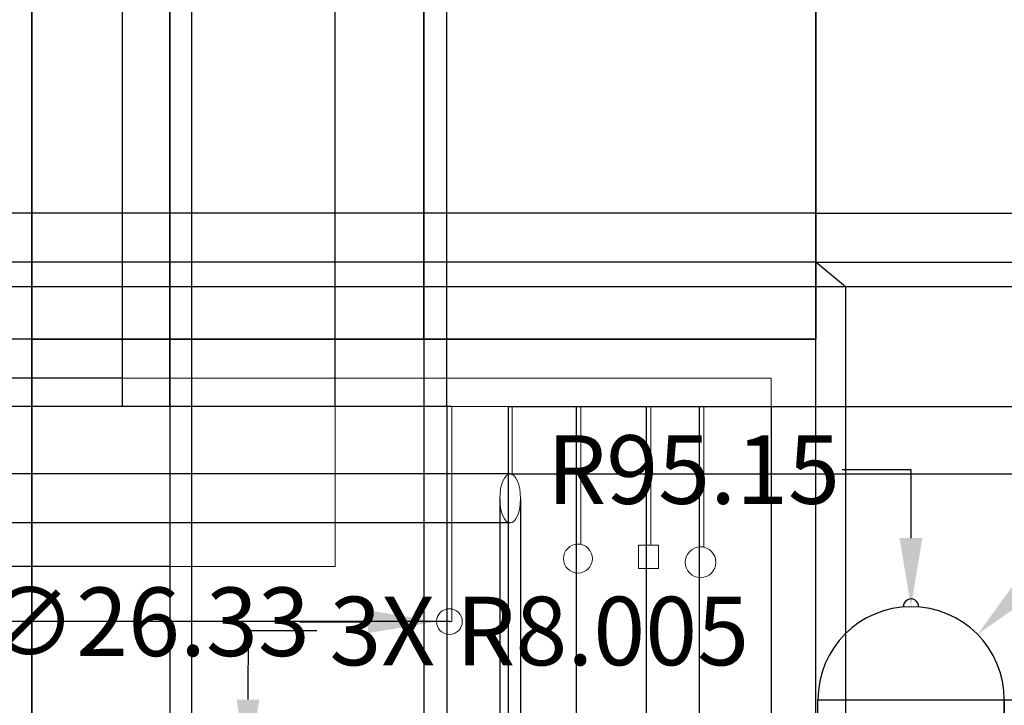
# Model space of a CAD drawing. Units: inches. Extents: x 600 to 5582, y -464 to 3142.
# Tile 4 of 9: x 1772 to 2777, y 1229 to 1928. Entities that reach past the tile are written whole.
import ezdxf

# ---------------------------------------------------------------- set-up
doc = ezdxf.new("R2010")
doc.units = ezdxf.units.IN
doc.header["$MEASUREMENT"] = 0
for name, color, linetype, lineweight in [('A-ANNO-DIMS', 2, 'Continuous', 18), ('A-ELEV', 7, 'Continuous', 35), ('A-ELEV-PATT', 252, 'Continuous', 13), ('A-EQPM', 4, 'Continuous', 25), ('A-FURN', 8, 'Continuous', 18)]:
    doc.layers.add(name, color=color, linetype=linetype, lineweight=lineweight)
doc.styles.get("Standard").update_dxf_attribs({"font": 'arial.ttf'})
doc.dimstyles.get("Standard").update_dxf_attribs({"dimtxt": 70, "dimasz": 70, "dimexe": 0.18, "dimexo": 0.0625, "dimgap": 0.09, "dimtad": 0, "dimtih": 1, "dimtoh": 1, "dimdec": 0, "dimzin": 0, "dimdsep": 46, "dimtxsty": 'Standard', "dimcen": 0.09, "dimadec": 0, "dimazin": 0, "dimtfac": 1, "dimtdec": 0, "dimtofl": 0, "dimtmove": 0, "dimatfit": 3, "dimfxl": 1, "dimtolj": 1, "dimtzin": 0, "dimarcsym": 0})

# ---------------------------------------------------------------- blocks, each defined once
blk = doc.blocks.new('*D22')
at = {"layer": 'A-ANNO-DIMS', "color": 0, "lineweight": -2, "transparency": 16777216}
for p, q in [((1149.2, 1725.8), (1149.2, 1795.8)), ((2615, 1655.8), (1149.1, 1655.8)), ((2584.7, 1602.4), (1149.1, 1602.4)), ((1149.2, 1532.4), (1149.2, 1462.4)), ((1149.2, 1462.4), (1079.2, 1462.4))]:
    blk.add_line(p, q, dxfattribs=at)
at = {"layer": 'A-ANNO-DIMS', "color": 0, "transparency": 16777216}
for points in [[(1137.6, 1725.8), (1160.9, 1725.8), (1149.2, 1655.8)], [(1137.6, 1532.4), (1160.9, 1532.4), (1149.2, 1602.4)]]:
    blk.add_solid(points, dxfattribs=at)
at = {"layer": 'Defpoints', "color": 0, "transparency": 16777216}
for p in [(2615, 1655.8), (1149.2, 1602.4), (2584.7, 1602.4)]:
    blk.add_point(p, dxfattribs=at)
at = {"layer": 'A-ANNO-DIMS', "color": 0, "transparency": 16777216, "insert": (967.8, 1462.4), "char_height": 70, "attachment_point": 5}
blk.add_mtext('\\A1;53.41', dxfattribs=at)
blk = doc.blocks.new('*D23')
at = {"layer": 'A-ANNO-DIMS', "color": 0, "lineweight": -2, "transparency": 16777216}
for p, q in [((1149.2, 1750.8), (1149.2, 1820.8)), ((1149.2, 1820.8), (1219.2, 1820.8)), ((2584.7, 1680.8), (1149.1, 1680.8)), ((2615, 1655.8), (1149.1, 1655.8)), ((1149.2, 1585.8), (1149.2, 1515.8))]:
    blk.add_line(p, q, dxfattribs=at)
at = {"layer": 'A-ANNO-DIMS', "color": 0, "transparency": 16777216}
for points in [[(1137.6, 1750.8), (1160.9, 1750.8), (1149.2, 1680.8)], [(1137.6, 1585.8), (1160.9, 1585.8), (1149.2, 1655.8)]]:
    blk.add_solid(points, dxfattribs=at)
at = {"layer": 'Defpoints', "color": 0, "transparency": 16777216}
for p in [(1149.2, 1680.8), (2584.7, 1680.8), (2615, 1655.8)]:
    blk.add_point(p, dxfattribs=at)
at = {"layer": 'A-ANNO-DIMS', "color": 0, "transparency": 16777216, "insert": (1270.3, 1820.8), "char_height": 70, "attachment_point": 5}
blk.add_mtext('\\A1;25', dxfattribs=at)
blk = doc.blocks.new('*D24')
at = {"layer": 'A-ANNO-DIMS', "color": 0, "lineweight": -2, "transparency": 16777216}
for p, q in [((1149.2, 1800.8), (1149.2, 1870.8)), ((1149.2, 1870.8), (1219.2, 1870.8)), ((2584.7, 1730.8), (1149.1, 1730.8)), ((2584.7, 1680.8), (1149.1, 1680.8)), ((1149.2, 1610.8), (1149.2, 1540.8))]:
    blk.add_line(p, q, dxfattribs=at)
at = {"layer": 'A-ANNO-DIMS', "color": 0, "transparency": 16777216}
for points in [[(1137.6, 1800.8), (1160.9, 1800.8), (1149.2, 1730.8)], [(1137.6, 1610.8), (1160.9, 1610.8), (1149.2, 1680.8)]]:
    blk.add_solid(points, dxfattribs=at)
at = {"layer": 'Defpoints', "color": 0, "transparency": 16777216}
for p in [(1149.2, 1730.8), (2584.7, 1730.8), (2584.7, 1680.8)]:
    blk.add_point(p, dxfattribs=at)
at = {"layer": 'A-ANNO-DIMS', "color": 0, "transparency": 16777216, "insert": (1269.4, 1870.8), "char_height": 70, "attachment_point": 5}
blk.add_mtext('\\A1;50', dxfattribs=at)
blk = doc.blocks.new('*D25')
at = {"layer": 'A-ANNO-DIMS', "color": 0, "lineweight": -2, "transparency": 16777216}
for p, q in [((2584.7, 1680.8), (2584.7, -233.3)), ((2615, 1655.8), (2615, -233.3)), ((2514.7, -233.1), (2444.7, -233.1)), ((2685, -233.1), (2755, -233.1))]:
    blk.add_line(p, q, dxfattribs=at)
at = {"layer": 'A-ANNO-DIMS', "color": 0, "transparency": 16777216}
for points in [[(2514.7, -221.4), (2514.7, -244.7), (2584.7, -233.1)], [(2685, -221.4), (2685, -244.7), (2615, -233.1)]]:
    blk.add_solid(points, dxfattribs=at)
at = {"layer": 'Defpoints', "color": 0, "transparency": 16777216}
for p in [(2584.7, 1680.8), (2615, 1655.8), (2615, -233.1)]:
    blk.add_point(p, dxfattribs=at)
at = {"layer": 'A-ANNO-DIMS', "color": 0, "transparency": 16777216, "insert": (2873.3, -233.1), "char_height": 70, "attachment_point": 5}
blk.add_mtext('\\A1;30.28', dxfattribs=at)
blk = doc.blocks.new('*D59')
at = {"layer": 'A-ANNO-DIMS', "color": 0, "lineweight": -2, "transparency": 16777216}
for p, q in [((2611.9, 1469.2), (2681.9, 1469.2)), ((2681.9, 1469.2), (2681.9, 1399.2)), ((2682, 1234), (2682.2, 1234)), ((2682.1, 1234), (2682.1, 1234.1))]:
    blk.add_line(p, q, dxfattribs=at)
at = {"layer": 'A-ANNO-DIMS', "color": 0, "transparency": 16777216}
blk.add_solid([(2693.6, 1399.2), (2670.3, 1399.2), (2682, 1329.2)], dxfattribs=at)
at = {"layer": 'Defpoints', "color": 0, "transparency": 16777216}
for p in [(2682, 1329.2), (2682.1, 1234)]:
    blk.add_point(p, dxfattribs=at)
at = {"layer": 'A-ANNO-DIMS', "color": 0, "transparency": 16777216, "insert": (2459.9, 1469.2), "char_height": 70, "attachment_point": 5}
blk.add_mtext('\\A1;R95.15', dxfattribs=at)
blk = doc.blocks.new('*D63')
at = {"layer": 'A-ANNO-DIMS', "color": 0, "lineweight": -2, "transparency": 16777216}
for p, q in [((2584.7, 2352.4), (1149.1, 2352.4)), ((1149.2, 2282.4), (1149.2, 2077.5)), ((1149.2, 1800.8), (1149.2, 2005.8)), ((2584.7, 1730.8), (1149.1, 1730.8))]:
    blk.add_line(p, q, dxfattribs=at)
at = {"layer": 'A-ANNO-DIMS', "color": 0, "transparency": 16777216}
for points in [[(1137.6, 2282.4), (1160.9, 2282.4), (1149.2, 2352.4)], [(1137.6, 1800.8), (1160.9, 1800.8), (1149.2, 1730.8)]]:
    blk.add_solid(points, dxfattribs=at)
at = {"layer": 'Defpoints', "color": 0, "transparency": 16777216}
for p in [(1149.2, 2352.4), (2584.7, 2352.4), (2584.7, 1730.8)]:
    blk.add_point(p, dxfattribs=at)
at = {"layer": 'A-ANNO-DIMS', "color": 0, "transparency": 16777216, "insert": (1149.2, 2041.6), "char_height": 70, "attachment_point": 5}
blk.add_mtext('\\A1;621.59', dxfattribs=at)
blk = doc.blocks.new('*D65')
at = {"layer": 'A-ANNO-DIMS', "color": 0, "lineweight": -2, "transparency": 16777216}
for p, q in [((1784.7, 2352.4), (1784.7, -233.3)), ((2184.7, 2352.4), (2184.7, -233.3)), ((1714.7, -233.1), (1644.7, -233.1)), ((2254.7, -233.1), (2324.7, -233.1))]:
    blk.add_line(p, q, dxfattribs=at)
at = {"layer": 'A-ANNO-DIMS', "color": 0, "transparency": 16777216}
for points in [[(1714.7, -221.4), (1714.7, -244.7), (1784.7, -233.1)], [(2254.7, -221.4), (2254.7, -244.7), (2184.7, -233.1)]]:
    blk.add_solid(points, dxfattribs=at)
at = {"layer": 'Defpoints', "color": 0, "transparency": 16777216}
for p in [(1784.7, 2352.4), (2184.7, 2352.4), (2184.7, -233.1)]:
    blk.add_point(p, dxfattribs=at)
at = {"layer": 'A-ANNO-DIMS', "color": 0, "transparency": 16777216, "insert": (1984.7, -233.1), "char_height": 70, "attachment_point": 5}
blk.add_mtext('\\A1;400.00', dxfattribs=at)
blk = doc.blocks.new('*D70')
at = {"layer": 'A-ANNO-DIMS', "color": 0, "lineweight": -2, "transparency": 16777216}
for p, q in [((1149.2, 1176.8), (1149.2, 1246.8)), ((1149.2, 1246.8), (1219.2, 1246.8)), ((2586.9, 1106.8), (1149.1, 1106.8)), ((2599.2, 1042.4), (1149.1, 1042.4)), ((1149.2, 972.4), (1149.2, 902.4))]:
    blk.add_line(p, q, dxfattribs=at)
at = {"layer": 'A-ANNO-DIMS', "color": 0, "transparency": 16777216}
for points in [[(1137.6, 1176.8), (1160.9, 1176.8), (1149.2, 1106.8)], [(1137.6, 972.4), (1160.9, 972.4), (1149.2, 1042.4)]]:
    blk.add_solid(points, dxfattribs=at)
at = {"layer": 'Defpoints', "color": 0, "transparency": 16777216}
for p in [(1149.2, 1106.8), (2586.9, 1106.8), (2599.2, 1042.4)]:
    blk.add_point(p, dxfattribs=at)
at = {"layer": 'A-ANNO-DIMS', "color": 0, "transparency": 16777216, "insert": (1337.3, 1246.8), "char_height": 70, "attachment_point": 5}
blk.add_mtext('\\A1;64.42', dxfattribs=at)
blk = doc.blocks.new('*D79')
at = {"layer": 'A-ANNO-DIMS', "color": 0, "lineweight": -2, "transparency": 16777216}
for p, q in [((1855.7, 2987.9), (1785.7, 2987.9)), ((1925.7, 1126.2), (1925.7, 2988.1)), ((1947.9, 1126.2), (1947.9, 2988.1)), ((2017.9, 2987.9), (2087.9, 2987.9))]:
    blk.add_line(p, q, dxfattribs=at)
at = {"layer": 'A-ANNO-DIMS', "color": 0, "transparency": 16777216}
for points in [[(1855.7, 2999.6), (1855.7, 2976.3), (1925.7, 2987.9)], [(2017.9, 2999.6), (2017.9, 2976.3), (1947.9, 2987.9)]]:
    blk.add_solid(points, dxfattribs=at)
at = {"layer": 'Defpoints', "color": 0, "transparency": 16777216}
for p in [(1947.9, 2987.9), (1925.7, 1126.1), (1947.9, 1126.1)]:
    blk.add_point(p, dxfattribs=at)
at = {"layer": 'A-ANNO-DIMS', "color": 0, "transparency": 16777216, "insert": (2234.2, 2987.9), "char_height": 70, "attachment_point": 5}
blk.add_mtext('\\A1;22.235', dxfattribs=at)
blk = doc.blocks.new('*D80')
at = {"layer": 'A-ANNO-DIMS', "color": 0, "lineweight": -2, "transparency": 16777216}
for p, q in [((1149.2, 1196.1), (1149.2, 1266.1)), ((1925.6, 1126.1), (1149.1, 1126.1)), ((1925.6, 1042.4), (1149.1, 1042.4)), ((1149.2, 972.4), (1149.2, 902.4))]:
    blk.add_line(p, q, dxfattribs=at)
at = {"layer": 'A-ANNO-DIMS', "color": 0, "transparency": 16777216}
for points in [[(1137.6, 1196.1), (1160.9, 1196.1), (1149.2, 1126.1)], [(1137.6, 972.4), (1160.9, 972.4), (1149.2, 1042.4)]]:
    blk.add_solid(points, dxfattribs=at)
at = {"layer": 'Defpoints', "color": 0, "transparency": 16777216}
for p in [(1149.2, 1126.1), (1925.7, 1126.1), (1925.7, 1042.4)]:
    blk.add_point(p, dxfattribs=at)
at = {"layer": 'A-ANNO-DIMS', "color": 0, "transparency": 16777216, "insert": (1149.2, 1084.3), "char_height": 70, "attachment_point": 5}
blk.add_mtext('\\A1;83.69', dxfattribs=at)
blk = doc.blocks.new('*D81')
at = {"layer": 'A-ANNO-DIMS', "color": 0, "lineweight": -2, "transparency": 16777216}
for p, q in [((5220.2, 1133.7), (5220.2, 1203.7)), ((5220.2, 1203.7), (5290.2, 1203.7)), ((2292.1, 1063.7), (5220.4, 1063.7)), ((2310.1, 1042.4), (5220.4, 1042.4)), ((5220.2, 972.4), (5220.2, 902.4))]:
    blk.add_line(p, q, dxfattribs=at)
at = {"layer": 'A-ANNO-DIMS', "color": 0, "transparency": 16777216}
for points in [[(5208.6, 1133.7), (5231.9, 1133.7), (5220.2, 1063.7)], [(5208.6, 972.4), (5231.9, 972.4), (5220.2, 1042.4)]]:
    blk.add_solid(points, dxfattribs=at)
at = {"layer": 'Defpoints', "color": 0, "transparency": 16777216}
for p in [(2292, 1063.7), (5220.2, 1063.7), (2310, 1042.4)]:
    blk.add_point(p, dxfattribs=at)
at = {"layer": 'A-ANNO-DIMS', "color": 0, "transparency": 16777216, "insert": (5409, 1203.7), "char_height": 70, "attachment_point": 5}
blk.add_mtext('\\A1;21.26', dxfattribs=at)
blk = doc.blocks.new('*D85')
at = {"layer": 'A-ANNO-DIMS', "color": 0, "lineweight": -2, "transparency": 16777216}
for p, q in [((5220.2, 1193.3), (5220.2, 1263.3)), ((5220.2, 1263.3), (5290.2, 1263.3)), ((2231.9, 1123.3), (5220.4, 1123.3)), ((2232.3, 1063.4), (5220.4, 1063.4)), ((5220.2, 993.4), (5220.2, 923.4))]:
    blk.add_line(p, q, dxfattribs=at)
at = {"layer": 'A-ANNO-DIMS', "color": 0, "transparency": 16777216}
for points in [[(5208.6, 1193.3), (5231.9, 1193.3), (5220.2, 1123.3)], [(5208.6, 993.4), (5231.9, 993.4), (5220.2, 1063.4)]]:
    blk.add_solid(points, dxfattribs=at)
at = {"layer": 'Defpoints', "color": 0, "transparency": 16777216}
for p in [(2231.8, 1123.3), (5220.2, 1123.3), (2232.2, 1063.4)]:
    blk.add_point(p, dxfattribs=at)
at = {"layer": 'A-ANNO-DIMS', "color": 0, "transparency": 16777216, "insert": (5408.5, 1263.3), "char_height": 70, "attachment_point": 5}
blk.add_mtext('\\A1;59.99', dxfattribs=at)
blk = doc.blocks.new('*D86')
at = {"layer": 'A-ANNO-DIMS', "color": 0, "lineweight": -2, "transparency": 16777216}
for p, q in [((1714.7, 2987.9), (1644.7, 2987.9)), ((1784.7, 1602.5), (1784.7, 2988.1)), ((1877.2, 1562.7), (1877.2, 2988.1)), ((1947.2, 2987.9), (2017.2, 2987.9))]:
    blk.add_line(p, q, dxfattribs=at)
at = {"layer": 'A-ANNO-DIMS', "color": 0, "transparency": 16777216}
for points in [[(1714.7, 2999.6), (1714.7, 2976.3), (1784.7, 2987.9)], [(1947.2, 2999.6), (1947.2, 2976.3), (1877.2, 2987.9)]]:
    blk.add_solid(points, dxfattribs=at)
at = {"layer": 'Defpoints', "color": 0, "transparency": 16777216}
for p in [(1877.2, 2987.9), (1784.7, 1602.4), (1877.2, 1562.6)]:
    blk.add_point(p, dxfattribs=at)
at = {"layer": 'A-ANNO-DIMS', "color": 0, "transparency": 16777216, "insert": (2135.4, 2987.9), "char_height": 70, "attachment_point": 5}
blk.add_mtext('\\A1;92.46', dxfattribs=at)
blk = doc.blocks.new('*D87')
at = {"layer": 'A-ANNO-DIMS', "color": 0, "lineweight": -2, "transparency": 16777216}
for p, q in [((1149.2, 1672.4), (1149.2, 1742.4)), ((1149.2, 1742.4), (1219.2, 1742.4)), ((1784.7, 1602.4), (1149.1, 1602.4)), ((1877.1, 1562.6), (1149.1, 1562.6)), ((1149.2, 1492.6), (1149.2, 1422.6))]:
    blk.add_line(p, q, dxfattribs=at)
at = {"layer": 'A-ANNO-DIMS', "color": 0, "transparency": 16777216}
for points in [[(1137.6, 1672.4), (1160.9, 1672.4), (1149.2, 1602.4)], [(1137.6, 1492.6), (1160.9, 1492.6), (1149.2, 1562.6)]]:
    blk.add_solid(points, dxfattribs=at)
at = {"layer": 'Defpoints', "color": 0, "transparency": 16777216}
for p in [(1149.2, 1602.4), (1784.7, 1602.4), (1877.2, 1562.6)]:
    blk.add_point(p, dxfattribs=at)
at = {"layer": 'A-ANNO-DIMS', "color": 0, "transparency": 16777216, "insert": (1337.3, 1742.4), "char_height": 70, "attachment_point": 5}
blk.add_mtext('\\A1;39.80', dxfattribs=at)
blk = doc.blocks.new('*D88')
at = {"layer": 'A-ANNO-DIMS', "color": 0, "lineweight": -2, "transparency": 16777216}
for p, q in [((1149.2, 1632.6), (1149.2, 1702.6)), ((1149.2, 1702.6), (1219.2, 1702.6)), ((1877.1, 1562.6), (1149.1, 1562.6)), ((1877.1, 1533.5), (1149.1, 1533.5)), ((1149.2, 1463.5), (1149.2, 1393.5))]:
    blk.add_line(p, q, dxfattribs=at)
at = {"layer": 'A-ANNO-DIMS', "color": 0, "transparency": 16777216}
for points in [[(1137.6, 1632.6), (1160.9, 1632.6), (1149.2, 1562.6)], [(1137.6, 1463.5), (1160.9, 1463.5), (1149.2, 1533.5)]]:
    blk.add_solid(points, dxfattribs=at)
at = {"layer": 'Defpoints', "color": 0, "transparency": 16777216}
for p in [(1149.2, 1562.6), (1877.2, 1562.6), (1877.2, 1533.5)]:
    blk.add_point(p, dxfattribs=at)
at = {"layer": 'A-ANNO-DIMS', "color": 0, "transparency": 16777216, "insert": (1365.2, 1702.6), "char_height": 70, "attachment_point": 5}
blk.add_mtext('\\A1;29.136', dxfattribs=at)
blk = doc.blocks.new('*D89')
at = {"layer": 'A-ANNO-DIMS', "color": 0, "lineweight": -2, "transparency": 16777216}
for p, q in [((1807.2, 2987.9), (1737.2, 2987.9)), ((1877.2, 1533.5), (1877.2, 2988.1)), ((1925.6, 1533.5), (1925.6, 2988.1)), ((1995.6, 2987.9), (2065.6, 2987.9))]:
    blk.add_line(p, q, dxfattribs=at)
at = {"layer": 'A-ANNO-DIMS', "color": 0, "transparency": 16777216}
for points in [[(1807.2, 2999.6), (1807.2, 2976.3), (1877.2, 2987.9)], [(1995.6, 2999.6), (1995.6, 2976.3), (1925.6, 2987.9)]]:
    blk.add_solid(points, dxfattribs=at)
at = {"layer": 'Defpoints', "color": 0, "transparency": 16777216}
for p in [(1925.6, 2987.9), (1877.2, 1533.5), (1925.6, 1533.5)]:
    blk.add_point(p, dxfattribs=at)
at = {"layer": 'A-ANNO-DIMS', "color": 0, "transparency": 16777216, "insert": (2185.1, 2987.9), "char_height": 70, "attachment_point": 5}
blk.add_mtext('\\A1;48.40', dxfattribs=at)
blk = doc.blocks.new('*D90')
at = {"layer": 'A-ANNO-DIMS', "color": 0, "lineweight": -2, "transparency": 16777216}
for p, q in [((1925.6, 1533.5), (1925.6, 2988.1)), ((1995.6, 2987.9), (2024.2, 2987.9)), ((2094.2, 1533.5), (2094.2, 2988.1)), ((2094.2, 2987.9), (2164.2, 2987.9))]:
    blk.add_line(p, q, dxfattribs=at)
at = {"layer": 'A-ANNO-DIMS', "color": 0, "transparency": 16777216}
for points in [[(1995.6, 2999.6), (1995.6, 2976.3), (1925.6, 2987.9)], [(2024.2, 2999.6), (2024.2, 2976.3), (2094.2, 2987.9)]]:
    blk.add_solid(points, dxfattribs=at)
at = {"layer": 'Defpoints', "color": 0, "transparency": 16777216}
for p in [(2094.2, 2987.9), (1925.6, 1533.5), (2094.2, 1533.5)]:
    blk.add_point(p, dxfattribs=at)
at = {"layer": 'A-ANNO-DIMS', "color": 0, "transparency": 16777216, "insert": (2306.2, 2987.9), "char_height": 70, "attachment_point": 5}
blk.add_mtext('\\A1;168.56', dxfattribs=at)
blk = doc.blocks.new('*D91')
at = {"layer": 'A-ANNO-DIMS', "color": 0, "lineweight": -2, "transparency": 16777216}
for p, q in [((2024.2, 2987.9), (1954.2, 2987.9)), ((2094.2, 1533.5), (2094.2, 2988.1)), ((2208.2, 1533.5), (2208.2, 2988.1)), ((2278.2, 2987.9), (2348.2, 2987.9))]:
    blk.add_line(p, q, dxfattribs=at)
at = {"layer": 'A-ANNO-DIMS', "color": 0, "transparency": 16777216}
for points in [[(2024.2, 2999.6), (2024.2, 2976.3), (2094.2, 2987.9)], [(2278.2, 2999.6), (2278.2, 2976.3), (2208.2, 2987.9)]]:
    blk.add_solid(points, dxfattribs=at)
at = {"layer": 'Defpoints', "color": 0, "transparency": 16777216}
for p in [(2208.2, 2987.9), (2094.2, 1533.5), (2208.2, 1533.5)]:
    blk.add_point(p, dxfattribs=at)
at = {"layer": 'A-ANNO-DIMS', "color": 0, "transparency": 16777216, "insert": (2490.3, 2987.9), "char_height": 70, "attachment_point": 5}
blk.add_mtext('\\A1;114.03', dxfattribs=at)
blk = doc.blocks.new('*D92')
at = {"layer": 'A-ANNO-DIMS', "color": 0, "lineweight": -2, "transparency": 16777216}
for p, q in [((2208.2, 1533.4), (2208.2, -233.3)), ((2271, 1533.4), (2271, -233.3)), ((2138.2, -233.1), (2068.2, -233.1)), ((2341, -233.1), (2411, -233.1))]:
    blk.add_line(p, q, dxfattribs=at)
at = {"layer": 'A-ANNO-DIMS', "color": 0, "transparency": 16777216}
for points in [[(2138.2, -221.4), (2138.2, -244.7), (2208.2, -233.1)], [(2341, -221.4), (2341, -244.7), (2271, -233.1)]]:
    blk.add_solid(points, dxfattribs=at)
at = {"layer": 'Defpoints', "color": 0, "transparency": 16777216}
for p in [(2208.2, 1533.5), (2271, 1533.5), (2271, -233.1)]:
    blk.add_point(p, dxfattribs=at)
at = {"layer": 'A-ANNO-DIMS', "color": 0, "transparency": 16777216, "insert": (2529.3, -233.1), "char_height": 70, "attachment_point": 5}
blk.add_mtext('\\A1;62.77', dxfattribs=at)
blk = doc.blocks.new('*D93')
at = {"layer": 'A-ANNO-DIMS', "color": 0, "lineweight": -2, "transparency": 16777216}
for p, q in [((2271, 1533.4), (2271, -233.3)), ((2340.4, 1533.4), (2340.4, -233.3)), ((2201, -233.1), (2131, -233.1)), ((2410.4, -233.1), (2480.4, -233.1))]:
    blk.add_line(p, q, dxfattribs=at)
at = {"layer": 'A-ANNO-DIMS', "color": 0, "transparency": 16777216}
for points in [[(2201, -221.4), (2201, -244.7), (2271, -233.1)], [(2410.4, -221.4), (2410.4, -244.7), (2340.4, -233.1)]]:
    blk.add_solid(points, dxfattribs=at)
at = {"layer": 'Defpoints', "color": 0, "transparency": 16777216}
for p in [(2271, 1533.5), (2340.4, 1533.5), (2340.4, -233.1)]:
    blk.add_point(p, dxfattribs=at)
at = {"layer": 'A-ANNO-DIMS', "color": 0, "transparency": 16777216, "insert": (2598.6, -233.1), "char_height": 70, "attachment_point": 5}
blk.add_mtext('\\A1;69.40', dxfattribs=at)
blk = doc.blocks.new('*D94')
at = {"layer": 'A-ANNO-DIMS', "color": 0, "lineweight": -2, "transparency": 16777216}
for p, q in [((2340.4, 1533.4), (2340.4, -233.3)), ((2411.7, 1533.4), (2411.7, -233.3)), ((2270.4, -233.1), (2200.4, -233.1)), ((2481.7, -233.1), (2551.7, -233.1))]:
    blk.add_line(p, q, dxfattribs=at)
at = {"layer": 'A-ANNO-DIMS', "color": 0, "transparency": 16777216}
for points in [[(2270.4, -221.4), (2270.4, -244.7), (2340.4, -233.1)], [(2481.7, -221.4), (2481.7, -244.7), (2411.7, -233.1)]]:
    blk.add_solid(points, dxfattribs=at)
at = {"layer": 'Defpoints', "color": 0, "transparency": 16777216}
for p in [(2340.4, 1533.5), (2411.7, 1533.5), (2411.7, -233.1)]:
    blk.add_point(p, dxfattribs=at)
at = {"layer": 'A-ANNO-DIMS', "color": 0, "transparency": 16777216, "insert": (2669.5, -233.1), "char_height": 70, "attachment_point": 5}
blk.add_mtext('\\A1;71.34', dxfattribs=at)
blk = doc.blocks.new('*D95')
at = {"layer": 'A-ANNO-DIMS', "color": 0, "lineweight": -2, "transparency": 16777216}
for p, q in [((2411.7, 1533.4), (2411.7, -233.3)), ((2465.8, 1533.4), (2465.8, -233.3)), ((2341.7, -233.1), (2271.7, -233.1)), ((2535.8, -233.1), (2605.8, -233.1))]:
    blk.add_line(p, q, dxfattribs=at)
at = {"layer": 'A-ANNO-DIMS', "color": 0, "transparency": 16777216}
for points in [[(2341.7, -221.4), (2341.7, -244.7), (2411.7, -233.1)], [(2535.8, -221.4), (2535.8, -244.7), (2465.8, -233.1)]]:
    blk.add_solid(points, dxfattribs=at)
at = {"layer": 'Defpoints', "color": 0, "transparency": 16777216}
for p in [(2411.7, 1533.5), (2465.8, 1533.5), (2465.8, -233.1)]:
    blk.add_point(p, dxfattribs=at)
at = {"layer": 'A-ANNO-DIMS', "color": 0, "transparency": 16777216, "insert": (2724, -233.1), "char_height": 70, "attachment_point": 5}
blk.add_mtext('\\A1;54.13', dxfattribs=at)
blk = doc.blocks.new('*D96')
at = {"layer": 'A-ANNO-DIMS', "color": 0, "lineweight": -2, "transparency": 16777216}
for p, q in [((2465.8, 1533.4), (2465.8, -233.3)), ((2539.2, 1533.4), (2539.2, -233.3)), ((2395.8, -233.1), (2325.8, -233.1)), ((2609.2, -233.1), (2679.2, -233.1))]:
    blk.add_line(p, q, dxfattribs=at)
at = {"layer": 'A-ANNO-DIMS', "color": 0, "transparency": 16777216}
for points in [[(2395.8, -221.4), (2395.8, -244.7), (2465.8, -233.1)], [(2609.2, -221.4), (2609.2, -244.7), (2539.2, -233.1)]]:
    blk.add_solid(points, dxfattribs=at)
at = {"layer": 'Defpoints', "color": 0, "transparency": 16777216}
for p in [(2465.8, 1533.5), (2539.2, 1533.5), (2539.2, -233.1)]:
    blk.add_point(p, dxfattribs=at)
at = {"layer": 'A-ANNO-DIMS', "color": 0, "transparency": 16777216, "insert": (2797.1, -233.1), "char_height": 70, "attachment_point": 5}
blk.add_mtext('\\A1;73.33', dxfattribs=at)
blk = doc.blocks.new('*D97')
at = {"layer": 'A-ANNO-DIMS', "color": 0, "lineweight": -2, "transparency": 16777216}
for p, q in [((1149.2, 1533.5), (1149.2, 1603.5)), ((1149.2, 1603.5), (1219.2, 1603.5)), ((1925.5, 1533.5), (1149.1, 1533.5)), ((1149.2, 1440.2), (1149.2, 1463.5)), ((1925.5, 1370.2), (1149.1, 1370.2))]:
    blk.add_line(p, q, dxfattribs=at)
at = {"layer": 'A-ANNO-DIMS', "color": 0, "transparency": 16777216}
for points in [[(1137.6, 1463.5), (1160.9, 1463.5), (1149.2, 1533.5)], [(1137.6, 1440.2), (1160.9, 1440.2), (1149.2, 1370.2)]]:
    blk.add_solid(points, dxfattribs=at)
at = {"layer": 'Defpoints', "color": 0, "transparency": 16777216}
for p in [(1149.2, 1533.5), (1925.6, 1533.5), (1925.6, 1370.2)]:
    blk.add_point(p, dxfattribs=at)
at = {"layer": 'A-ANNO-DIMS', "color": 0, "transparency": 16777216, "insert": (1354.6, 1603.5), "char_height": 70, "attachment_point": 5}
blk.add_mtext('\\A1;163.31', dxfattribs=at)
blk = doc.blocks.new('*D98')
at = {"layer": 'A-ANNO-DIMS', "color": 0, "lineweight": -2, "transparency": 16777216}
for p, q in [((2213.4, 1533.5), (1149.1, 1533.5)), ((1149.2, 1463.5), (1149.2, 1459.6)), ((1149.2, 1384), (1149.2, 1387.9)), ((2210.8, 1314), (1149.1, 1314))]:
    blk.add_line(p, q, dxfattribs=at)
at = {"layer": 'A-ANNO-DIMS', "color": 0, "transparency": 16777216}
for points in [[(1137.6, 1463.5), (1160.9, 1463.5), (1149.2, 1533.5)], [(1137.6, 1384), (1160.9, 1384), (1149.2, 1314)]]:
    blk.add_solid(points, dxfattribs=at)
at = {"layer": 'Defpoints', "color": 0, "transparency": 16777216}
for p in [(2213.5, 1533.5), (1149.2, 1314), (2210.8, 1314)]:
    blk.add_point(p, dxfattribs=at)
at = {"layer": 'A-ANNO-DIMS', "color": 0, "transparency": 16777216, "insert": (1149.2, 1423.8), "char_height": 70, "attachment_point": 5}
blk.add_mtext('\\A1;219.47', dxfattribs=at)
blk = doc.blocks.new('*D99')
at = {"layer": 'A-ANNO-DIMS', "color": 0, "lineweight": -2, "transparency": 16777216}
for p, q in [((5220.2, 1603.5), (5220.2, 1673.5)), ((2271, 1533.5), (5220.4, 1533.5)), ((2273, 1464.8), (5220.4, 1464.8)), ((5220.2, 1394.8), (5220.2, 1324.8)), ((5220.2, 1324.8), (5150.2, 1324.8))]:
    blk.add_line(p, q, dxfattribs=at)
at = {"layer": 'A-ANNO-DIMS', "color": 0, "transparency": 16777216}
for points in [[(5208.6, 1603.5), (5231.9, 1603.5), (5220.2, 1533.5)], [(5208.6, 1394.8), (5231.9, 1394.8), (5220.2, 1464.8)]]:
    blk.add_solid(points, dxfattribs=at)
at = {"layer": 'Defpoints', "color": 0, "transparency": 16777216}
for p in [(2271, 1533.5), (2272.9, 1464.8), (5220.2, 1464.8)]:
    blk.add_point(p, dxfattribs=at)
at = {"layer": 'A-ANNO-DIMS', "color": 0, "transparency": 16777216, "insert": (5038.6, 1324.8), "char_height": 70, "attachment_point": 5}
blk.add_mtext('\\A1;68.71', dxfattribs=at)
blk = doc.blocks.new('*D100')
at = {"layer": 'A-ANNO-DIMS', "color": 0, "lineweight": -2, "transparency": 16777216}
for p, q in [((2262.3, 1439.7), (2262.3, -233.3)), ((2283.5, 1439.7), (2283.5, -233.3)), ((2192.3, -233.1), (2122.3, -233.1)), ((2353.5, -233.1), (2423.5, -233.1))]:
    blk.add_line(p, q, dxfattribs=at)
at = {"layer": 'A-ANNO-DIMS', "color": 0, "transparency": 16777216}
for points in [[(2192.3, -221.4), (2192.3, -244.7), (2262.3, -233.1)], [(2353.5, -221.4), (2353.5, -244.7), (2283.5, -233.1)]]:
    blk.add_solid(points, dxfattribs=at)
at = {"layer": 'Defpoints', "color": 0, "transparency": 16777216}
for p in [(2262.3, 1439.7), (2283.5, 1439.7), (2283.5, -233.1)]:
    blk.add_point(p, dxfattribs=at)
at = {"layer": 'A-ANNO-DIMS', "color": 0, "transparency": 16777216, "insert": (2569.4, -233.1), "char_height": 70, "attachment_point": 5}
blk.add_mtext('\\A1;21.136', dxfattribs=at)
blk = doc.blocks.new('*D101')
at = {"layer": 'A-ANNO-DIMS', "color": 0, "lineweight": -2, "transparency": 16777216}
for p, q in [((1149.2, 1534.8), (1149.2, 1604.8)), ((2272.8, 1464.8), (1149.1, 1464.8)), ((2272.8, 1414.7), (1149.1, 1414.7)), ((1149.2, 1344.7), (1149.2, 1274.7)), ((1149.2, 1274.7), (1079.2, 1274.7))]:
    blk.add_line(p, q, dxfattribs=at)
at = {"layer": 'A-ANNO-DIMS', "color": 0, "transparency": 16777216}
for points in [[(1137.6, 1534.8), (1160.9, 1534.8), (1149.2, 1464.8)], [(1137.6, 1344.7), (1160.9, 1344.7), (1149.2, 1414.7)]]:
    blk.add_solid(points, dxfattribs=at)
at = {"layer": 'Defpoints', "color": 0, "transparency": 16777216}
for p in [(2272.9, 1464.8), (1149.2, 1414.7), (2272.9, 1414.7)]:
    blk.add_point(p, dxfattribs=at)
at = {"layer": 'A-ANNO-DIMS', "color": 0, "transparency": 16777216, "insert": (961.1, 1274.7), "char_height": 70, "attachment_point": 5}
blk.add_mtext('\\A1;50.13', dxfattribs=at)
blk = doc.blocks.new('*D103')
at = {"layer": 'A-ANNO-DIMS', "color": 0, "lineweight": -2, "transparency": 16777216}
for p, q in [((2849.5, 1399.2), (2799.7, 1350)), ((2919.5, 1399.2), (2849.5, 1399.2)), ((2682, 1234), (2682.2, 1234)), ((2682.1, 1234), (2682.1, 1234.1))]:
    blk.add_line(p, q, dxfattribs=at)
at = {"layer": 'A-ANNO-DIMS', "color": 0, "transparency": 16777216}
blk.add_solid([(2791.5, 1358.3), (2807.9, 1341.7), (2749.9, 1300.9)], dxfattribs=at)
at = {"layer": 'Defpoints', "color": 0, "transparency": 16777216}
for p in [(2749.9, 1300.9), (2682.1, 1234)]:
    blk.add_point(p, dxfattribs=at)
at = {"layer": 'A-ANNO-DIMS', "color": 0, "transparency": 16777216, "insert": (3071.5, 1399.2), "char_height": 70, "attachment_point": 5}
blk.add_mtext('\\A1;R95.15', dxfattribs=at)
blk = doc.blocks.new('*D104')
at = {"layer": 'A-ANNO-DIMS', "color": 0, "lineweight": -2, "transparency": 16777216}
for p, q in [((1786.6, 1212.4), (1856.6, 1212.4)), ((1856.6, 1212.4), (1916.6, 1176.4)), ((2004.9, 1123.3), (2005.1, 1123.3)), ((2005, 1123.3), (2005, 1123.4))]:
    blk.add_line(p, q, dxfattribs=at)
at = {"layer": 'A-ANNO-DIMS', "color": 0, "transparency": 16777216}
blk.add_solid([(1922.6, 1186.4), (1910.6, 1166.4), (1976.6, 1140.4)], dxfattribs=at)
at = {"layer": 'Defpoints', "color": 0, "transparency": 16777216}
for p in [(1976.6, 1140.4), (2005, 1123.3)]:
    blk.add_point(p, dxfattribs=at)
at = {"layer": 'A-ANNO-DIMS', "color": 0, "transparency": 16777216, "insert": (1559.9, 1212.4), "char_height": 70, "attachment_point": 5}
blk.add_mtext('\\A1;3X R33.04', dxfattribs=at)
blk = doc.blocks.new('*D105')
at = {"layer": 'A-ANNO-DIMS', "color": 0, "lineweight": -2, "transparency": 16777216}
for p, q in [((2005.5, 1304.4), (2005.2, 1234.4)), ((2075.5, 1304.4), (2005.5, 1304.4)), ((2004.9, 1156.4), (2005.1, 1156.4)), ((2005, 1156.3), (2005, 1156.5))]:
    blk.add_line(p, q, dxfattribs=at)
at = {"layer": 'A-ANNO-DIMS', "color": 0, "transparency": 16777216}
blk.add_solid([(1993.6, 1234.4), (2016.9, 1234.4), (2005, 1164.4)], dxfattribs=at)
at = {"layer": 'Defpoints', "color": 0, "transparency": 16777216}
for p in [(2005, 1164.4), (2005, 1156.4)]:
    blk.add_point(p, dxfattribs=at)
at = {"layer": 'A-ANNO-DIMS', "color": 0, "transparency": 16777216, "insert": (2302.6, 1304.4), "char_height": 70, "attachment_point": 5}
blk.add_mtext('\\A1;3X R8.005', dxfattribs=at)
blk = doc.blocks.new('*D106')
at = {"layer": 'A-ANNO-DIMS', "color": 0, "lineweight": -2, "transparency": 16777216}
for p, q in [((2057.7, 1313.8), (2127.7, 1313.9)), ((2210.7, 1314), (2210.9, 1314)), ((2210.8, 1313.9), (2210.8, 1314.1))]:
    blk.add_line(p, q, dxfattribs=at)
at = {"layer": 'A-ANNO-DIMS', "color": 0, "transparency": 16777216}
blk.add_solid([(2127.7, 1325.5), (2127.7, 1302.2), (2197.7, 1314)], dxfattribs=at)
at = {"layer": 'Defpoints', "color": 0, "transparency": 16777216}
for p in [(2197.7, 1314), (2224, 1314)]:
    blk.add_point(p, dxfattribs=at)
at = {"layer": 'A-ANNO-DIMS', "color": 0, "transparency": 16777216, "insert": (1901.4, 1313.8), "char_height": 70, "attachment_point": 5}
blk.add_mtext('\\A1;∅26.33', dxfattribs=at)

msp = doc.modelspace()

# ---------------------------------------------------------------- hatches: boundary and pattern name
at = {"layer": 'A-ELEV-PATT'}
h = msp.add_hatch(dxfattribs=at)
h.set_pattern_fill('CROSS', color=256, scale=100)
h.paths.add_polyline_path([(1759.7485, 2327.4212), (1409.7485, 2327.4212), (1409.7485, 1967.4212), (1759.7485, 1967.4212)])
h.paths.add_polyline_path([(1759.7485, 1952.4212), (1409.7485, 1952.4212), (1409.7485, 1567.4212), (1759.7485, 1567.4212)])
h.paths.add_polyline_path([(1759.7485, 1552.4212), (1409.7485, 1552.4212), (1409.7485, 1167.4212), (1759.7485, 1167.4212)])
h.paths.add_polyline_path([(1759.7485, 1152.4212), (1409.7485, 1152.4212), (1409.7485, 767.4212), (1759.7485, 767.4212)])
h.paths.add_polyline_path([(1759.7485, 752.4212), (1409.7485, 752.4212), (1409.7485, 367.4212), (1759.7485, 367.4212)])
h.paths.add_polyline_path([(1759.7485, 352.4212), (1409.7485, 352.4212), (1409.7485, 142.4212), (1759.7485, 142.4212)])
h.paths.add_polyline_path([(3759.7485, 1977.4212), (3409.7485, 1977.4212), (3409.7485, 1627.4212), (3759.7485, 1627.4212)])
h.paths.add_polyline_path([(3714.7508, 1954.858, -1), (3750.8891, 1954.858, -1)], flags=16)
h.paths.add_polyline_path([(3759.7485, 2327.4212), (3409.7485, 2327.4212), (3409.7485, 2002.4212), (3759.7485, 2002.4212)])
h.paths.add_polyline_path([(4159.7485, 2327.4212), (3809.7485, 2327.4212), (3809.7485, 2002.4212), (4159.7485, 2002.4212)])
h.paths.add_polyline_path([(4159.7485, 1977.4212), (3809.7485, 1977.4212), (3813.5467, 1954.858, -1), (3849.685, 1954.858, -1), (3813.5467, 1954.858), (3809.7485, 1627.4212), (4159.7485, 1627.4212)])
h.paths.add_polyline_path([(4559.7485, 2327.4212), (4184.7485, 2327.4212), (4184.7485, 2002.4212), (4559.7485, 2002.4212)])
h.paths.add_polyline_path([(4559.7485, 1977.4212), (4184.7485, 1977.4212), (4184.7485, 1627.4212), (4559.7485, 1627.4212)])
h.paths.add_polyline_path([(4517.0704, 1954.858, -1), (4553.2087, 1954.858, -1)], flags=16)
h.paths.add_polyline_path([(4959.7485, 2327.4212), (4609.7485, 2327.4212), (4609.7485, 2002.4212), (4959.7485, 2002.4212)])
h.paths.add_polyline_path([(4959.7485, 1977.4212), (4609.7485, 1977.4212), (4609.7485, 1627.4212), (4959.7485, 1627.4212)])
h.paths.add_polyline_path([(4619.5464, 1954.858, -1), (4655.6847, 1954.858, -1)], flags=16)

# ---------------------------------------------------------------- linework, layer by layer
at = {"layer": 'A-ELEV'}
for points in [[(1784.7485, 2.4212), (1784.7485, 2352.4212), (1384.7485, 2352.4212), (1409.7485, 2327.4212), (1759.7485, 2327.4212), (1409.7485, 2327.4212), (1409.7485, 127.4212)], [(1759.7485, 127.4212), (1759.7485, 2327.4212), (1784.7485, 2352.4212), (2184.7485, 2352.4212), (2184.7485, 1602.4212)], [(1784.7485, 1602.4212), (2584.7485, 1602.4212), (2584.7485, 2352.4212)]]:
    msp.add_lwpolyline(points, dxfattribs=at)
at = {"layer": 'A-EQPM'}
msp.add_line((2584.7485, 1730.8271), (3384.7485, 1730.8271), dxfattribs=at)
for points in [[(3384.7485, 1680.8271), (3356.5781, 1655.8271), (2615.026, 1655.8271), (2584.7485, 1680.8271)], [(2586.9456, 1106.8415), (2586.9456, 1234.0488), (2777.2556, 1234.0488), (2777.2556, 1106.8415)], [(2777.2556, 1234.0488), (2947.8448, 1234.0488), (2947.8448, 1211.9616), (2777.2556, 1211.9616)]]:
    msp.add_lwpolyline(points, close=True, dxfattribs=at)
for centre, radius, start, end in [((2682.1006, 1329.2037), 7.8768, 357.627886, 182.372114), ((2682.1006, 1234.0488), 95.155, 0, 180)]:
    msp.add_arc(centre, radius, start, end, dxfattribs=at)
at = {"layer": 'A-FURN'}
for points in [[(1877.2057, 1562.623), (2539.1643, 1562.623), (2539.1643, 1533.4874), (1877.2057, 1533.4874)], [(2403.7898, 1392.0949), (2424.3362, 1392.0949), (2424.3362, 1368.0808), (2403.7898, 1368.0808)]]:
    msp.add_lwpolyline(points, close=True, dxfattribs=at)
msp.add_lwpolyline([(1925.6025, 1533.4874), (1925.6025, 1370.1726), (2094.1593, 1370.1726), (2094.1593, 1533.4874), (2208.185, 1533.4874), (2208.185, 1314.0217), (2213.4889, 1314.0217), (2213.4889, 1533.4874), (2270.9593, 1533.4874), (2270.9593, 1464.7817), (2274.8457, 1464.7817), (2274.8457, 1533.4874), (2340.3598, 1533.4874), (2340.3598, 1392.9272), (2345.079, 1392.9272), (2345.079, 1533.4874), (2411.7034, 1533.4874), (2411.7034, 1392.0949), (2416.4226, 1392.0949), (2416.4226, 1533.4874), (2465.8357, 1533.4874), (2465.8357, 1390.1529), (2465.8357, 1390.1529), (2470.555, 1390.1529), (2470.555, 1533.4874)], dxfattribs=at)
for centre, radius in [((2342.0372, 1378.2705), 14.7524), ((2467.2613, 1374.5225), 15.6583), ((2210.837, 1314.0217), 13.1649)]:
    msp.add_circle(centre, radius, dxfattribs=at)
msp.add_ellipse((2272.9025, 1439.718), major_axis=(0, -25.0637), ratio=0.421642887, dxfattribs=at)

# ---------------------------------------------------------------- dimensions: what is measured, and where the dimension line sits
at = {"layer": 'A-ANNO-DIMS'}
for base, p1, p2, override, picture, middle in [((1877.2057, 2987.9212), (1784.7485, 1602.4212), (1877.2057, 1562.623), {"dimdec": 2, "dimlfac": 1, "dimrnd": 0, "dimzin": 0, "dimdsep": 46, "dimlunit": 2}, '*D86', (2135.3789, 2987.9212)), ((1925.6025, 2987.9212), (1877.2057, 1533.4874), (1925.6025, 1533.4874), {"dimdec": 2, "dimlfac": 1, "dimrnd": 0, "dimzin": 0, "dimdsep": 46, "dimlunit": 2}, '*D89', (2185.0889, 2987.9212)), ((1947.9344, 2987.9212), (1925.6996, 1126.1128), (1947.9344, 1126.1128), {"dimdec": 3, "dimlfac": 1, "dimrnd": 0, "dimzin": 0, "dimdsep": 46, "dimlunit": 2}, '*D79', (2234.1841, 2987.9212)), ((2094.1593, 2987.9212), (1925.6025, 1533.4874), (2094.1593, 1533.4874), {"dimdec": 2, "dimlfac": 1, "dimrnd": 0, "dimzin": 0, "dimdsep": 46, "dimlunit": 2}, '*D90', (2306.2308, 2987.9212)), ((2208.185, 2987.9212), (2094.1593, 1533.4874), (2208.185, 1533.4874), {"dimdec": 2, "dimlfac": 1, "dimrnd": 0, "dimzin": 0, "dimdsep": 46, "dimlunit": 2}, '*D91', (2490.2805, 2987.9212)), ((2184.7485, -233.0788), (1784.7485, 2352.4212), (2184.7485, 2352.4212), {"dimdec": 2, "dimlfac": 1, "dimrnd": 0, "dimzin": 0, "dimdsep": 46, "dimlunit": 2}, '*D65', (1984.7485, -233.0788)), ((2615.026, -233.0788), (2584.7485, 1680.8271), (2615.026, 1655.8271), {"dimdec": 2, "dimlfac": 1, "dimrnd": 0, "dimzin": 0, "dimdsep": 46, "dimlunit": 2}, '*D25', (2873.2709, -233.0788)), ((2270.9593, -233.0788), (2208.185, 1533.4874), (2270.9593, 1533.4874), {"dimdec": 2, "dimlfac": 1, "dimrnd": 0, "dimzin": 0, "dimdsep": 46, "dimlunit": 2}, '*D92', (2529.3474, -233.0788)), ((2340.3598, -233.0788), (2270.9593, 1533.4874), (2340.3598, 1533.4874), {"dimdec": 2, "dimlfac": 1, "dimrnd": 0, "dimzin": 0, "dimdsep": 46, "dimlunit": 2}, '*D93', (2598.6285, -233.0788)), ((2411.7034, -233.0788), (2340.3598, 1533.4874), (2411.7034, 1533.4874), {"dimdec": 2, "dimlfac": 1, "dimrnd": 0, "dimzin": 0, "dimdsep": 46, "dimlunit": 2}, '*D94', (2669.4707, -233.0788)), ((2465.8357, -233.0788), (2411.7034, 1533.4874), (2465.8357, 1533.4874), {"dimdec": 2, "dimlfac": 1, "dimrnd": 0, "dimzin": 0, "dimdsep": 46, "dimlunit": 2}, '*D95', (2724.0328, -233.0788)), ((2539.1643, -233.0788), (2465.8357, 1533.4874), (2539.1643, 1533.4874), {"dimdec": 2, "dimlfac": 1, "dimrnd": 0, "dimzin": 0, "dimdsep": 46, "dimlunit": 2}, '*D96', (2797.0749, -233.0788)), ((2283.4705, -233.0788), (2262.3346, 1439.718), (2283.4705, 1439.718), {"dimdec": 3, "dimlfac": 1, "dimrnd": 0, "dimzin": 0, "dimdsep": 46, "dimlunit": 2}, '*D100', (2569.4336, -233.0788))]:
    dim = msp.add_linear_dim(base=base, p1=p1, p2=p2, dimstyle='Standard', override=override, dxfattribs=at)
    dim.commit()
    dim.dimension.update_dxf_attribs({"geometry": picture, "text_midpoint": middle})
for base, p1, p2, override, picture, middle in [((1149.2485, 2352.4212), (2584.7485, 1730.8271), (2584.7485, 2352.4212), {"dimdec": 2, "dimlfac": 1, "dimrnd": 0, "dimzin": 0, "dimdsep": 46, "dimlunit": 2}, '*D63', (1149.2485, 2041.6241)), ((1149.2485, 1730.8271), (2584.7485, 1680.8271), (2584.7485, 1730.8271), {"dimdec": 0, "dimlfac": 1, "dimrnd": 0, "dimzin": 0, "dimdsep": 46, "dimlunit": 2}, '*D24', (1269.3555, 1870.8271)), ((1149.2485, 1680.8271), (2615.026, 1655.8271), (2584.7485, 1680.8271), {"dimdec": 0, "dimlfac": 1, "dimrnd": 0, "dimzin": 0, "dimdsep": 46, "dimlunit": 2}, '*D23', (1270.3344, 1820.8271)), ((1149.2485, 1602.4212), (2615.026, 1655.8271), (2584.7485, 1602.4212), {"dimdec": 2, "dimlfac": 1, "dimrnd": 0, "dimzin": 0, "dimdsep": 46, "dimlunit": 2}, '*D22', (967.8079, 1462.4212)), ((1149.2485, 1602.4212), (1877.2057, 1562.623), (1784.7485, 1602.4212), {"dimdec": 2, "dimlfac": 1, "dimrnd": 0, "dimzin": 0, "dimdsep": 46, "dimlunit": 2}, '*D87', (1337.3023, 1742.4212)), ((1149.2485, 1562.623), (1877.2057, 1533.4874), (1877.2057, 1562.623), {"dimdec": 3, "dimlfac": 1, "dimrnd": 0, "dimzin": 0, "dimdsep": 46, "dimlunit": 2}, '*D88', (1365.2116, 1702.623)), ((5220.2485, 1464.7817), (2270.9593, 1533.4874), (2272.9025, 1464.7817), {"dimdec": 2, "dimlfac": 1, "dimrnd": 0, "dimzin": 0, "dimdsep": 46, "dimlunit": 2}, '*D99', (5038.6169, 1324.7817)), ((1149.2485, 1533.4874), (1925.6025, 1370.1726), (1925.6025, 1533.4874), {"dimdec": 2, "dimlfac": 1, "dimrnd": 0, "dimzin": 0, "dimdsep": 46, "dimlunit": 2}, '*D97', (1354.5875, 1603.4874)), ((1149.2485, 1414.6543), (2272.9025, 1464.7817), (2272.9025, 1414.6543), {"dimdec": 2, "dimlfac": 1, "dimrnd": 0, "dimzin": 0, "dimdsep": 46, "dimlunit": 2}, '*D101', (961.0514, 1274.6543)), ((1149.2485, 1314.0217), (2213.4889, 1533.4874), (2210.837, 1314.0217), {"dimdec": 2, "dimlfac": 1, "dimrnd": 0, "dimzin": 0, "dimdsep": 46, "dimlunit": 2}, '*D98', (1149.2485, 1423.7545)), ((5220.2485, 1123.3472), (2232.228, 1063.362), (2231.8275, 1123.3472), {"dimdec": 2, "dimlfac": 1, "dimrnd": 0, "dimzin": 0, "dimdsep": 46, "dimlunit": 2}, '*D85', (5408.5172, 1263.3472)), ((1149.2485, 1106.8415), (2599.2497, 1042.42), (2586.9456, 1106.8415), {"dimdec": 2, "dimlfac": 1, "dimrnd": 0, "dimzin": 0, "dimdsep": 46, "dimlunit": 2}, '*D70', (1337.2784, 1246.8415)), ((1149.2485, 1126.1128), (1925.6996, 1042.4212), (1925.6996, 1126.1128), {"dimdec": 2, "dimlfac": 1, "dimrnd": 0, "dimzin": 0, "dimdsep": 46, "dimlunit": 2}, '*D80', (1149.2485, 1084.267)), ((5220.2485, 1063.682), (2310.0444, 1042.4212), (2292.0448, 1063.682), {"dimdec": 2, "dimlfac": 1, "dimrnd": 0, "dimzin": 0, "dimdsep": 46, "dimlunit": 2}, '*D81', (5409.0186, 1203.682))]:
    dim = msp.add_linear_dim(base=base, p1=p1, p2=p2, angle=90, dimstyle='Standard', override=override, dxfattribs=at)
    dim.commit()
    dim.dimension.update_dxf_attribs({"geometry": picture, "text_midpoint": middle})
for center, mpoint, picture, middle in [((2682.1006, 1234.0488), (2681.9998, 1329.2037), '*D59', (2459.8958, 1469.2036)), ((2682.10062, 1234.04876), (2749.85675, 1300.85875), '*D103', (3071.5009, 1399.15523))]:
    dim = msp.add_radius_dim(center=center, mpoint=mpoint, dimstyle='Standard', override={"dimdec": 2, "dimlfac": 1, "dimrnd": 0, "dimzin": 0, "dimdsep": 46, "dimlunit": 2}, dxfattribs=at)
    dim.commit()
    dim.dimension.update_dxf_attribs({"geometry": picture, "text_midpoint": middle})
for center, mpoint, override, picture, middle in [((2004.9671, 1156.3876), (2004.9945, 1164.3922), {"dimdec": 3, "dimlfac": 1, "dimrnd": 0, "dimzin": 0, "dimdsep": 46, "dimlunit": 2}, '*D105', (2302.6098, 1304.3914)), ((2004.9671, 1123.3472), (1976.6406, 1140.3555), {"dimdec": 2, "dimlfac": 1, "dimrnd": 0, "dimzin": 0, "dimdsep": 46, "dimlunit": 2}, '*D104', (1559.8844, 1212.4236))]:
    dim = msp.add_radius_dim(center=center, mpoint=mpoint, text='3X <>', dimstyle='Standard', override=override, dxfattribs=at)
    dim.commit()
    dim.dimension.update_dxf_attribs({"geometry": picture, "text_midpoint": middle})
dim = msp.add_diameter_dim_2p(p1=(2224.0018, 1314.0439), p2=(2197.6721, 1313.9994), dimstyle='Standard', override={"dimdec": 2, "dimlfac": 1, "dimrnd": 0, "dimzin": 0, "dimdsep": 46, "dimlunit": 2}, dxfattribs=at)
dim.commit()
dim.dimension.update_dxf_attribs({"geometry": '*D106', "text_midpoint": (2057.6723, 1313.7633)})

doc.saveas('drawing.dxf')
